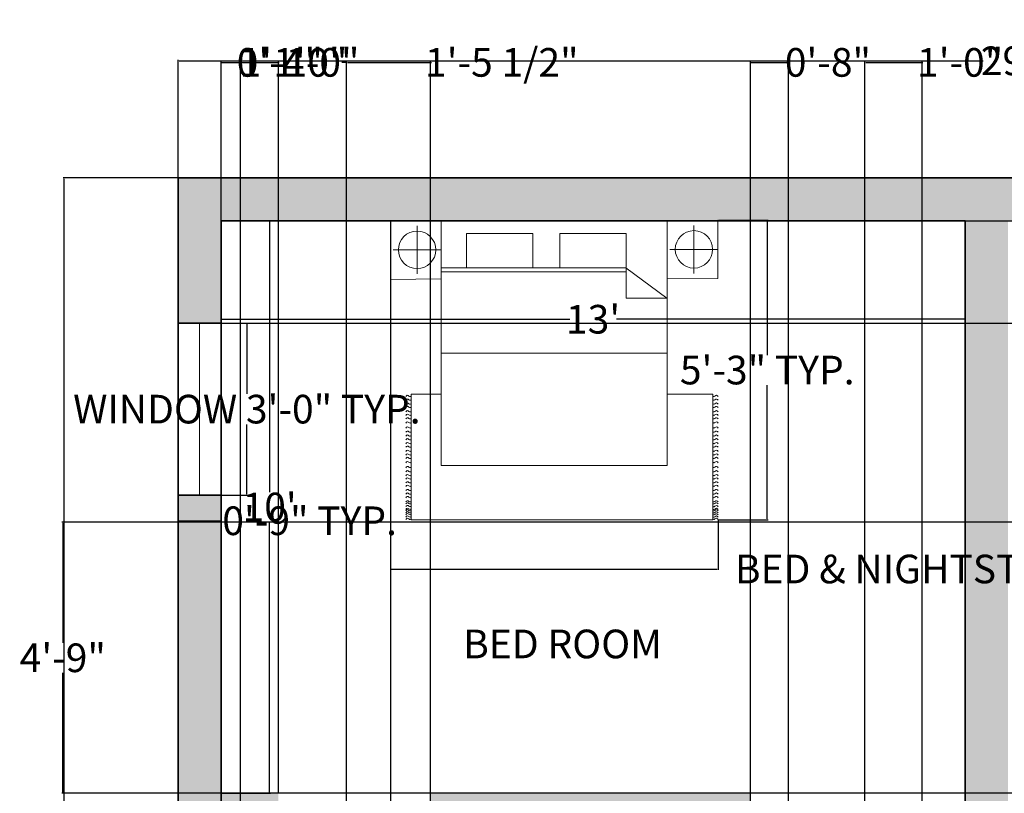
# Model space of a CAD drawing. Units: inches. Extents: x 1174 to 1615, y 3112 to 3628.
# Tile 4 of 6: x 1183 to 1390, y 3466 to 3628. Entities that reach past the tile are written whole.
import ezdxf

# ---------------------------------------------------------------- set-up
doc = ezdxf.new("R2010")
doc.units = ezdxf.units.IN
doc.header["$MEASUREMENT"] = 0
doc.layers.get('0').update_dxf_attribs({"color": 250})
for name, color, linetype, lineweight in [('A-ANNO-DIMS', 2, 'Continuous', 18), ('A-AREA-IDEN', 7, 'Continuous', 25), ('A-FURN', 8, 'Continuous', 13), ('A-GLAZ', 4, 'Continuous', 18), ('A-WALL', 7, 'Continuous', 35)]:
    doc.layers.add(name, color=color, linetype=linetype, lineweight=lineweight)
doc.layers.add('A-WALL-PATT', color=18, linetype='Continuous', lineweight=13, true_color=0x000000)
doc.styles.get("Standard").update_dxf_attribs({"font": 'arial.ttf'})
doc.dimstyles.get("Standard").update_dxf_attribs({"dimtxt": 6, "dimasz": 0.18, "dimexe": 0.18, "dimexo": 0.0625, "dimgap": 0.09, "dimtad": 0, "dimtih": 1, "dimtoh": 1, "dimdec": 1, "dimzin": 0, "dimdsep": 46, "dimlunit": 3, "dimtxsty": 'Standard', "dimcen": 0.09, "dimadec": 0, "dimazin": 0, "dimtfac": 1, "dimtdec": 1, "dimtofl": 0, "dimtmove": 0, "dimatfit": 3, "dimfxl": 1, "dimtolj": 1, "dimtzin": 0, "dimarcsym": 0})

# ---------------------------------------------------------------- blocks, each defined once
blk = doc.blocks.new('*D3')
at = {"layer": 'A-ANNO-DIMS', "color": 0, "lineweight": -2, "transparency": 16777216}
for p, q in [((1216.66, 3595.09), (1216.66, 3619.74)), ((1216.84, 3619.56), (1385.43, 3619.56)), ((1564.48, 3619.56), (1395.9, 3619.56)), ((1564.66, 3595.09), (1564.66, 3619.74))]:
    blk.add_line(p, q, dxfattribs=at)
at = {"layer": 'A-ANNO-DIMS', "color": 0, "transparency": 16777216}
for points in [[(1216.84, 3619.59), (1216.84, 3619.53), (1216.66, 3619.56)], [(1564.48, 3619.59), (1564.48, 3619.53), (1564.66, 3619.56)]]:
    blk.add_solid(points, dxfattribs=at)
at = {"layer": 'Defpoints', "color": 0, "transparency": 16777216}
for p in [(1564.66, 3619.56), (1216.66, 3595.03), (1564.66, 3595.03)]:
    blk.add_point(p, dxfattribs=at)
at = {"layer": 'A-ANNO-DIMS', "color": 0, "transparency": 16777216, "insert": (1390.66, 3619.56), "char_height": 6, "attachment_point": 5}
blk.add_mtext("\\A1;29'", dxfattribs=at)
blk = doc.blocks.new('*D4')
at = {"layer": 'A-ANNO-DIMS', "color": 0, "lineweight": -2, "transparency": 16777216}
for p, q in [((1216.6, 3595.03), (1192.51, 3595.03)), ((1192.69, 3594.85), (1192.69, 3388.18)), ((1192.69, 3175.21), (1192.69, 3381.87)), ((1216.6, 3175.03), (1192.51, 3175.03))]:
    blk.add_line(p, q, dxfattribs=at)
at = {"layer": 'A-ANNO-DIMS', "color": 0, "transparency": 16777216}
for points in [[(1192.66, 3594.85), (1192.72, 3594.85), (1192.69, 3595.03)], [(1192.66, 3175.21), (1192.72, 3175.21), (1192.69, 3175.03)]]:
    blk.add_solid(points, dxfattribs=at)
at = {"layer": 'Defpoints', "color": 0, "transparency": 16777216}
for p in [(1216.66, 3595.03), (1192.69, 3175.03), (1216.66, 3175.03)]:
    blk.add_point(p, dxfattribs=at)
at = {"layer": 'A-ANNO-DIMS', "color": 0, "transparency": 16777216, "insert": (1192.69, 3385.03), "char_height": 6, "attachment_point": 5}
blk.add_mtext("\\A1;35'", dxfattribs=at)
blk = doc.blocks.new('*D5')
at = {"layer": 'A-ANNO-DIMS', "color": 0, "lineweight": -2, "transparency": 16777216}
for p, q in [((1225.73, 3586.03), (1236.02, 3586.03)), ((1235.84, 3585.85), (1235.84, 3529.18)), ((1235.84, 3466.21), (1235.84, 3522.88)), ((1225.73, 3466.03), (1236.02, 3466.03))]:
    blk.add_line(p, q, dxfattribs=at)
at = {"layer": 'A-ANNO-DIMS', "color": 0, "transparency": 16777216}
for points in [[(1235.81, 3585.85), (1235.87, 3585.85), (1235.84, 3586.03)], [(1235.81, 3466.21), (1235.87, 3466.21), (1235.84, 3466.03)]]:
    blk.add_solid(points, dxfattribs=at)
at = {"layer": 'Defpoints', "color": 0, "transparency": 16777216}
for p in [(1225.66, 3586.03), (1225.66, 3466.03), (1235.84, 3466.03)]:
    blk.add_point(p, dxfattribs=at)
at = {"layer": 'A-ANNO-DIMS', "color": 0, "transparency": 16777216, "insert": (1235.84, 3526.03), "char_height": 6, "attachment_point": 5}
blk.add_mtext("\\A1;10'", dxfattribs=at)
blk = doc.blocks.new('*D6')
at = {"layer": 'A-ANNO-DIMS', "color": 0, "lineweight": -2, "transparency": 16777216}
for p, q in [((1225.66, 3585.97), (1225.66, 3565.21)), ((1381.66, 3585.97), (1381.66, 3565.21)), ((1225.84, 3565.39), (1298.76, 3565.39)), ((1381.48, 3565.39), (1308.56, 3565.39))]:
    blk.add_line(p, q, dxfattribs=at)
at = {"layer": 'A-ANNO-DIMS', "color": 0, "transparency": 16777216}
for points in [[(1225.84, 3565.42), (1225.84, 3565.36), (1225.66, 3565.39)], [(1381.48, 3565.42), (1381.48, 3565.36), (1381.66, 3565.39)]]:
    blk.add_solid(points, dxfattribs=at)
at = {"layer": 'Defpoints', "color": 0, "transparency": 16777216}
for p in [(1225.66, 3586.03), (1381.66, 3586.03), (1381.66, 3565.39)]:
    blk.add_point(p, dxfattribs=at)
at = {"layer": 'A-ANNO-DIMS', "color": 0, "transparency": 16777216, "insert": (1303.66, 3565.39), "char_height": 6, "attachment_point": 5}
blk.add_mtext("\\A1;13'", dxfattribs=at)
blk = doc.blocks.new('BED-DOUBLE-WITH-NIGHTSTANDS')
for p, q in [((5.6, 61.61), (5.6, 51.56)), ((63.65, 61.72), (63.65, 51.66)), ((10.63, 56.59), (0.57, 56.59)), ((68.68, 56.69), (58.62, 56.69)), ((49.39, 52.82), (10.63, 52.82)), ((49.44, 52), (10.63, 52)), ((49.39, 52.82), (58, 46.47)), ((49.44, 52.82), (49.44, 46.47)), ((49.44, 46.47), (58, 46.47)), ((58.05, 34.96), (10.63, 34.96)), ((4.35, 0), (4.35, 26.37)), ((4.35, 26.37), (10.65, 26.37)), ((58.05, 26.37), (67.59, 26.37)), ((67.59, 26.37), (67.59, 0)), ((67.59, 0), (4.35, 0))]:
    blk.add_line(p, q)
for points in [[(0, 50.39), (10.63, 50.5), (10.63, 62.68), (0, 62.58)], [(58.05, 62.68), (58.05, 11.36), (10.63, 11.36), (10.63, 62.68)], [(58.05, 50.5), (68.68, 50.6), (68.68, 62.78), (58.05, 62.68)], [(29.88, 59.98), (29.88, 52.82), (15.98, 52.82), (15.98, 59.98)], [(49.44, 59.98), (49.44, 52.82), (35.55, 52.82), (35.55, 59.98)]]:
    blk.add_lwpolyline(points, close=True)
for centre in [(5.6, 56.59), (63.65, 56.69)]:
    blk.add_circle(centre, 3.92)
for points, knots in [([(3.23, 25.83), (3.32, 25.96), (3.52, 26.2), (3.86, 25.96), (4.14, 25.78), (4.29, 25.89), (4.35, 25.94)], [0, 0, 0, 0, 0.400747, 0.791423, 1.067667, 1.29709, 1.29709, 1.29709, 1.29709]), ([(3.23, 25.06), (3.32, 25.18), (3.52, 25.42), (3.86, 25.18), (4.14, 25.01), (4.29, 25.11), (4.35, 25.16)], [0, 0, 0, 0, 0.400747, 0.791423, 1.067667, 1.29709, 1.29709, 1.29709, 1.29709]), ([(68.71, 25.83), (68.61, 25.96), (68.42, 26.2), (68.08, 25.96), (67.8, 25.78), (67.65, 25.89), (67.58, 25.94)], [0, 0, 0, 0, 0.400747, 0.791423, 1.067667, 1.29709, 1.29709, 1.29709, 1.29709]), ([(68.71, 25.06), (68.61, 25.18), (68.42, 25.42), (68.08, 25.18), (67.8, 25.01), (67.65, 25.11), (67.58, 25.16)], [0, 0, 0, 0, 0.400747, 0.791423, 1.067667, 1.29709, 1.29709, 1.29709, 1.29709]), ([(3.23, 24.24), (3.32, 24.36), (3.52, 24.6), (3.86, 24.36), (4.14, 24.19), (4.29, 24.3), (4.35, 24.34)], [0, 0, 0, 0, 0.400747, 0.791423, 1.067667, 1.29709, 1.29709, 1.29709, 1.29709]), ([(3.23, 23.51), (3.32, 23.63), (3.52, 23.87), (3.86, 23.63), (4.14, 23.46), (4.29, 23.57), (4.35, 23.62)], [0, 0, 0, 0, 0.400747, 0.791423, 1.067667, 1.29709, 1.29709, 1.29709, 1.29709]), ([(3.23, 22.63), (3.32, 22.75), (3.52, 22.99), (3.86, 22.75), (4.14, 22.58), (4.29, 22.69), (4.35, 22.73)], [0, 0, 0, 0, 0.400747, 0.791423, 1.067667, 1.29709, 1.29709, 1.29709, 1.29709]), ([(68.71, 24.24), (68.61, 24.36), (68.42, 24.6), (68.08, 24.36), (67.8, 24.19), (67.65, 24.3), (67.58, 24.34)], [0, 0, 0, 0, 0.400747, 0.791423, 1.067667, 1.29709, 1.29709, 1.29709, 1.29709]), ([(68.71, 23.51), (68.61, 23.63), (68.42, 23.87), (68.08, 23.63), (67.8, 23.46), (67.65, 23.57), (67.58, 23.62)], [0, 0, 0, 0, 0.400747, 0.791423, 1.067667, 1.29709, 1.29709, 1.29709, 1.29709]), ([(68.71, 22.63), (68.61, 22.75), (68.42, 22.99), (68.08, 22.75), (67.8, 22.58), (67.65, 22.69), (67.58, 22.73)], [0, 0, 0, 0, 0.400747, 0.791423, 1.067667, 1.29709, 1.29709, 1.29709, 1.29709]), ([(3.23, 21.88), (3.32, 22), (3.52, 22.24), (3.86, 22), (4.14, 21.83), (4.29, 21.93), (4.35, 21.98)], [0, 0, 0, 0, 0.400747, 0.791423, 1.067667, 1.29709, 1.29709, 1.29709, 1.29709]), ([(3.23, 21.15), (3.32, 21.27), (3.52, 21.51), (3.86, 21.27), (4.14, 21.1), (4.29, 21.21), (4.35, 21.25)], [0, 0, 0, 0, 0.400747, 0.791423, 1.067667, 1.29709, 1.29709, 1.29709, 1.29709]), ([(68.71, 21.88), (68.61, 22), (68.42, 22.24), (68.08, 22), (67.8, 21.83), (67.65, 21.93), (67.58, 21.98)], [0, 0, 0, 0, 0.400747, 0.791423, 1.067667, 1.29709, 1.29709, 1.29709, 1.29709]), ([(68.71, 21.15), (68.61, 21.27), (68.42, 21.51), (68.08, 21.27), (67.8, 21.1), (67.65, 21.21), (67.58, 21.25)], [0, 0, 0, 0, 0.400747, 0.791423, 1.067667, 1.29709, 1.29709, 1.29709, 1.29709]), ([(3.23, 20.27), (3.32, 20.39), (3.52, 20.63), (3.86, 20.39), (4.14, 20.22), (4.29, 20.32), (4.35, 20.37)], [0, 0, 0, 0, 0.400747, 0.791423, 1.067667, 1.29709, 1.29709, 1.29709, 1.29709]), ([(3.23, 19.23), (3.32, 19.35), (3.52, 19.59), (3.86, 19.35), (4.14, 19.18), (4.29, 19.29), (4.35, 19.33)], [0, 0, 0, 0, 0.400747, 0.791423, 1.067667, 1.29709, 1.29709, 1.29709, 1.29709]), ([(3.23, 18.35), (3.32, 18.47), (3.52, 18.71), (3.86, 18.47), (4.14, 18.3), (4.29, 18.4), (4.35, 18.45)], [0, 0, 0, 0, 0.400747, 0.791423, 1.067667, 1.29709, 1.29709, 1.29709, 1.29709]), ([(68.71, 20.27), (68.61, 20.39), (68.42, 20.63), (68.08, 20.39), (67.8, 20.22), (67.65, 20.32), (67.58, 20.37)], [0, 0, 0, 0, 0.400747, 0.791423, 1.067667, 1.29709, 1.29709, 1.29709, 1.29709]), ([(68.71, 19.23), (68.61, 19.35), (68.42, 19.59), (68.08, 19.35), (67.8, 19.18), (67.65, 19.29), (67.58, 19.33)], [0, 0, 0, 0, 0.400747, 0.791423, 1.067667, 1.29709, 1.29709, 1.29709, 1.29709]), ([(68.71, 18.35), (68.61, 18.47), (68.42, 18.71), (68.08, 18.47), (67.8, 18.3), (67.65, 18.4), (67.58, 18.45)], [0, 0, 0, 0, 0.400747, 0.791423, 1.067667, 1.29709, 1.29709, 1.29709, 1.29709]), ([(3.23, 17.53), (3.32, 17.65), (3.52, 17.89), (3.86, 17.65), (4.14, 17.48), (4.29, 17.59), (4.35, 17.64)], [0, 0, 0, 0, 0.400747, 0.791423, 1.067667, 1.29709, 1.29709, 1.29709, 1.29709]), ([(3.23, 16.76), (3.32, 16.88), (3.52, 17.12), (3.86, 16.88), (4.14, 16.7), (4.29, 16.81), (4.35, 16.86)], [0, 0, 0, 0, 0.400747, 0.791423, 1.067667, 1.29709, 1.29709, 1.29709, 1.29709]), ([(68.71, 17.53), (68.61, 17.65), (68.42, 17.89), (68.08, 17.65), (67.8, 17.48), (67.65, 17.59), (67.58, 17.64)], [0, 0, 0, 0, 0.400747, 0.791423, 1.067667, 1.29709, 1.29709, 1.29709, 1.29709]), ([(68.71, 16.76), (68.61, 16.88), (68.42, 17.12), (68.08, 16.88), (67.8, 16.7), (67.65, 16.81), (67.58, 16.86)], [0, 0, 0, 0, 0.400747, 0.791423, 1.067667, 1.29709, 1.29709, 1.29709, 1.29709]), ([(3.23, 15.94), (3.32, 16.06), (3.52, 16.3), (3.86, 16.06), (4.14, 15.89), (4.29, 15.99), (4.35, 16.04)], [0, 0, 0, 0, 0.400747, 0.791423, 1.067667, 1.29709, 1.29709, 1.29709, 1.29709]), ([(3.23, 15.21), (3.32, 15.33), (3.52, 15.57), (3.86, 15.33), (4.14, 15.16), (4.29, 15.27), (4.35, 15.32)], [0, 0, 0, 0, 0.400747, 0.791423, 1.067667, 1.29709, 1.29709, 1.29709, 1.29709]), ([(3.23, 14.33), (3.32, 14.45), (3.52, 14.69), (3.86, 14.45), (4.14, 14.28), (4.29, 14.38), (4.35, 14.43)], [0, 0, 0, 0, 0.400747, 0.791423, 1.067667, 1.29709, 1.29709, 1.29709, 1.29709]), ([(68.71, 15.94), (68.61, 16.06), (68.42, 16.3), (68.08, 16.06), (67.8, 15.89), (67.65, 15.99), (67.58, 16.04)], [0, 0, 0, 0, 0.400747, 0.791423, 1.067667, 1.29709, 1.29709, 1.29709, 1.29709]), ([(68.71, 15.21), (68.61, 15.33), (68.42, 15.57), (68.08, 15.33), (67.8, 15.16), (67.65, 15.27), (67.58, 15.32)], [0, 0, 0, 0, 0.400747, 0.791423, 1.067667, 1.29709, 1.29709, 1.29709, 1.29709]), ([(68.71, 14.33), (68.61, 14.45), (68.42, 14.69), (68.08, 14.45), (67.8, 14.28), (67.65, 14.38), (67.58, 14.43)], [0, 0, 0, 0, 0.400747, 0.791423, 1.067667, 1.29709, 1.29709, 1.29709, 1.29709]), ([(3.23, 13.58), (3.32, 13.7), (3.52, 13.94), (3.86, 13.7), (4.14, 13.53), (4.29, 13.63), (4.35, 13.68)], [0, 0, 0, 0, 0.400747, 0.791423, 1.067667, 1.29709, 1.29709, 1.29709, 1.29709]), ([(3.23, 12.85), (3.32, 12.97), (3.52, 13.21), (3.86, 12.97), (4.14, 12.8), (4.29, 12.9), (4.35, 12.95)], [0, 0, 0, 0, 0.400747, 0.791423, 1.067667, 1.29709, 1.29709, 1.29709, 1.29709]), ([(68.71, 13.58), (68.61, 13.7), (68.42, 13.94), (68.08, 13.7), (67.8, 13.53), (67.65, 13.63), (67.58, 13.68)], [0, 0, 0, 0, 0.400747, 0.791423, 1.067667, 1.29709, 1.29709, 1.29709, 1.29709]), ([(68.71, 12.85), (68.61, 12.97), (68.42, 13.21), (68.08, 12.97), (67.8, 12.8), (67.65, 12.9), (67.58, 12.95)], [0, 0, 0, 0, 0.400747, 0.791423, 1.067667, 1.29709, 1.29709, 1.29709, 1.29709]), ([(3.23, 11.97), (3.32, 12.09), (3.52, 12.33), (3.86, 12.09), (4.14, 11.92), (4.29, 12.02), (4.35, 12.07)], [0, 0, 0, 0, 0.400747, 0.791423, 1.067667, 1.29709, 1.29709, 1.29709, 1.29709]), ([(3.23, 10.93), (3.32, 11.05), (3.52, 11.29), (3.86, 11.05), (4.14, 10.88), (4.29, 10.99), (4.35, 11.03)], [0, 0, 0, 0, 0.400747, 0.791423, 1.067667, 1.29709, 1.29709, 1.29709, 1.29709]), ([(68.71, 11.97), (68.61, 12.09), (68.42, 12.33), (68.08, 12.09), (67.8, 11.92), (67.65, 12.02), (67.58, 12.07)], [0, 0, 0, 0, 0.400747, 0.791423, 1.067667, 1.29709, 1.29709, 1.29709, 1.29709]), ([(68.71, 10.93), (68.61, 11.05), (68.42, 11.29), (68.08, 11.05), (67.8, 10.88), (67.65, 10.99), (67.58, 11.03)], [0, 0, 0, 0, 0.400747, 0.791423, 1.067667, 1.29709, 1.29709, 1.29709, 1.29709]), ([(3.23, 10.05), (3.32, 10.17), (3.52, 10.41), (3.86, 10.17), (4.14, 10), (4.29, 10.1), (4.35, 10.15)], [0, 0, 0, 0, 0.400747, 0.791423, 1.067667, 1.29709, 1.29709, 1.29709, 1.29709]), ([(3.23, 9.23), (3.32, 9.35), (3.52, 9.59), (3.86, 9.35), (4.14, 9.18), (4.29, 9.29), (4.35, 9.34)], [0, 0, 0, 0, 0.400747, 0.791423, 1.067667, 1.29709, 1.29709, 1.29709, 1.29709]), ([(3.23, 8.54), (3.32, 8.66), (3.52, 8.9), (3.86, 8.66), (4.14, 8.49), (4.29, 8.6), (4.35, 8.65)], [0, 0, 0, 0, 0.400747, 0.791423, 1.067667, 1.29709, 1.29709, 1.29709, 1.29709]), ([(68.71, 10.05), (68.61, 10.17), (68.42, 10.41), (68.08, 10.17), (67.8, 10), (67.65, 10.1), (67.58, 10.15)], [0, 0, 0, 0, 0.400747, 0.791423, 1.067667, 1.29709, 1.29709, 1.29709, 1.29709]), ([(68.71, 9.23), (68.61, 9.35), (68.42, 9.59), (68.08, 9.35), (67.8, 9.18), (67.65, 9.29), (67.58, 9.34)], [0, 0, 0, 0, 0.400747, 0.791423, 1.067667, 1.29709, 1.29709, 1.29709, 1.29709]), ([(68.71, 8.54), (68.61, 8.66), (68.42, 8.9), (68.08, 8.66), (67.8, 8.49), (67.65, 8.6), (67.58, 8.65)], [0, 0, 0, 0, 0.400747, 0.791423, 1.067667, 1.29709, 1.29709, 1.29709, 1.29709]), ([(3.23, 7.73), (3.32, 7.85), (3.52, 8.09), (3.86, 7.85), (4.14, 7.68), (4.29, 7.78), (4.35, 7.83)], [0, 0, 0, 0, 0.400747, 0.791423, 1.067667, 1.29709, 1.29709, 1.29709, 1.29709]), ([(3.23, 7), (3.32, 7.12), (3.52, 7.36), (3.86, 7.12), (4.14, 6.95), (4.29, 7.05), (4.35, 7.1)], [0, 0, 0, 0, 0.400747, 0.791423, 1.067667, 1.29709, 1.29709, 1.29709, 1.29709]), ([(3.23, 6.12), (3.32, 6.24), (3.52, 6.48), (3.86, 6.24), (4.14, 6.06), (4.29, 6.17), (4.35, 6.22)], [0, 0, 0, 0, 0.400747, 0.791423, 1.067667, 1.29709, 1.29709, 1.29709, 1.29709]), ([(68.71, 7.73), (68.61, 7.85), (68.42, 8.09), (68.08, 7.85), (67.8, 7.68), (67.65, 7.78), (67.58, 7.83)], [0, 0, 0, 0, 0.400747, 0.791423, 1.067667, 1.29709, 1.29709, 1.29709, 1.29709]), ([(68.71, 7), (68.61, 7.12), (68.42, 7.36), (68.08, 7.12), (67.8, 6.95), (67.65, 7.05), (67.58, 7.1)], [0, 0, 0, 0, 0.400747, 0.791423, 1.067667, 1.29709, 1.29709, 1.29709, 1.29709]), ([(68.71, 6.12), (68.61, 6.24), (68.42, 6.48), (68.08, 6.24), (67.8, 6.06), (67.65, 6.17), (67.58, 6.22)], [0, 0, 0, 0, 0.400747, 0.791423, 1.067667, 1.29709, 1.29709, 1.29709, 1.29709]), ([(3.23, 5.36), (3.32, 5.49), (3.52, 5.73), (3.86, 5.49), (4.14, 5.31), (4.29, 5.42), (4.35, 5.47)], [0, 0, 0, 0, 0.400747, 0.791423, 1.067667, 1.29709, 1.29709, 1.29709, 1.29709]), ([(3.23, 4.64), (3.32, 4.76), (3.52, 5), (3.86, 4.76), (4.14, 4.58), (4.29, 4.69), (4.35, 4.74)], [0, 0, 0, 0, 0.400747, 0.791423, 1.067667, 1.29709, 1.29709, 1.29709, 1.29709]), ([(68.71, 5.36), (68.61, 5.49), (68.42, 5.73), (68.08, 5.49), (67.8, 5.31), (67.65, 5.42), (67.58, 5.47)], [0, 0, 0, 0, 0.400747, 0.791423, 1.067667, 1.29709, 1.29709, 1.29709, 1.29709]), ([(68.71, 4.64), (68.61, 4.76), (68.42, 5), (68.08, 4.76), (67.8, 4.59), (67.66, 4.69), (67.59, 4.73)], [0, 0, 0, 0, 0.400747, 0.791423, 1.067667, 1.283686, 1.283686, 1.283686, 1.283686]), ([(3.23, 3.75), (3.32, 3.88), (3.52, 4.11), (3.86, 3.88), (4.14, 3.7), (4.29, 3.81), (4.35, 3.86)], [0, 0, 0, 0, 0.400747, 0.791423, 1.067667, 1.29709, 1.29709, 1.29709, 1.29709]), ([(3.23, 3.32), (3.32, 3.45), (3.51, 3.7), (3.86, 3.44), (4.14, 3.27), (4.29, 3.38), (4.35, 3.43)], [0, 0, 0, 0, 0.407265, 0.802015, 1.07826, 1.307683, 1.307683, 1.307683, 1.307683]), ([(3.23, 2.76), (3.32, 2.88), (3.52, 3.12), (3.86, 2.88), (4.14, 2.71), (4.29, 2.81), (4.35, 2.86)], [0, 0, 0, 0, 0.400747, 0.791423, 1.067667, 1.29709, 1.29709, 1.29709, 1.29709]), ([(3.23, 2.18), (3.32, 2.31), (3.52, 2.55), (3.86, 2.31), (4.14, 2.13), (4.29, 2.24), (4.35, 2.29)], [0, 0, 0, 0, 0.400747, 0.791423, 1.067667, 1.29709, 1.29709, 1.29709, 1.29709]), ([(3.23, 1.88), (3.32, 2), (3.52, 2.24), (3.86, 2), (4.14, 1.82), (4.29, 1.93), (4.35, 1.98)], [0, 0, 0, 0, 0.400747, 0.791423, 1.067667, 1.29709, 1.29709, 1.29709, 1.29709]), ([(68.71, 3.75), (68.61, 3.88), (68.42, 4.11), (68.08, 3.88), (67.8, 3.7), (67.66, 3.8), (67.59, 3.85)], [0, 0, 0, 0, 0.400747, 0.791423, 1.067667, 1.283686, 1.283686, 1.283686, 1.283686]), ([(68.71, 3.32), (68.61, 3.45), (68.42, 3.69), (68.08, 3.45), (67.8, 3.27), (67.66, 3.38), (67.59, 3.42)], [0, 0, 0, 0, 0.402903, 0.794912, 1.071156, 1.287177, 1.287177, 1.287177, 1.287177]), ([(68.71, 2.73), (68.61, 2.85), (68.42, 3.09), (68.08, 2.85), (67.8, 2.68), (67.66, 2.78), (67.59, 2.82)], [0, 0, 0, 0, 0.400747, 0.791423, 1.067667, 1.283686, 1.283686, 1.283686, 1.283686]), ([(68.71, 2.16), (68.61, 2.28), (68.42, 2.52), (68.08, 2.28), (67.8, 2.11), (67.66, 2.21), (67.59, 2.25)], [0, 0, 0, 0, 0.400747, 0.791423, 1.067667, 1.283686, 1.283686, 1.283686, 1.283686]), ([(68.71, 1.85), (68.61, 1.97), (68.42, 2.21), (68.08, 1.97), (67.8, 1.8), (67.66, 1.9), (67.59, 1.94)], [0, 0, 0, 0, 0.400747, 0.791423, 1.067667, 1.283686, 1.283686, 1.283686, 1.283686]), ([(3.23, 1.46), (3.32, 1.58), (3.52, 1.82), (3.86, 1.58), (4.14, 1.4), (4.29, 1.51), (4.35, 1.56)], [0, 0, 0, 0, 0.400747, 0.791423, 1.067667, 1.29709, 1.29709, 1.29709, 1.29709]), ([(3.23, 1.06), (3.32, 1.18), (3.52, 1.42), (3.86, 1.18), (4.14, 1.01), (4.29, 1.11), (4.35, 1.16)], [0, 0, 0, 0, 0.400747, 0.791423, 1.067667, 1.29709, 1.29709, 1.29709, 1.29709]), ([(3.23, 0.57), (3.32, 0.7), (3.52, 0.93), (3.86, 0.7), (4.14, 0.52), (4.29, 0.63), (4.35, 0.68)], [0, 0, 0, 0, 0.400747, 0.791423, 1.067667, 1.29709, 1.29709, 1.29709, 1.29709]), ([(3.23, 0.07), (3.32, 0.19), (3.52, 0.43), (3.86, 0.19), (4.14, 0.02), (4.29, 0.13), (4.35, 0.18)], [0, 0, 0, 0, 0.400747, 0.791423, 1.067667, 1.29709, 1.29709, 1.29709, 1.29709]), ([(68.71, 1.43), (68.61, 1.55), (68.42, 1.79), (68.08, 1.55), (67.8, 1.38), (67.65, 1.48), (67.58, 1.53)], [0, 0, 0, 0, 0.400747, 0.791423, 1.067667, 1.29709, 1.29709, 1.29709, 1.29709]), ([(68.71, 1.03), (68.61, 1.15), (68.42, 1.39), (68.08, 1.15), (67.8, 0.98), (67.65, 1.09), (67.58, 1.13)], [0, 0, 0, 0, 0.400747, 0.791423, 1.067667, 1.29709, 1.29709, 1.29709, 1.29709]), ([(68.71, 0.55), (68.61, 0.67), (68.42, 0.91), (68.08, 0.67), (67.8, 0.49), (67.65, 0.6), (67.58, 0.65)], [0, 0, 0, 0, 0.400747, 0.791423, 1.067667, 1.29709, 1.29709, 1.29709, 1.29709]), ([(68.71, 0.07), (68.61, 0.19), (68.42, 0.43), (68.08, 0.19), (67.8, 0.02), (67.65, 0.13), (67.58, 0.18)], [0, 0, 0, 0, 0.400747, 0.791423, 1.067667, 1.29709, 1.29709, 1.29709, 1.29709])]:
    blk.add_open_spline(points, degree=3, knots=knots)
blk = doc.blocks.new('WINDOW-36IN')
for p, q in [((-4.5, -36), (-4.5, 0)), ((0, 0), (0, -36)), ((4.5, 0), (4.5, -36))]:
    blk.add_line(p, q)
blk = doc.blocks.new('*D26')
at = {"layer": 'A-ANNO-DIMS', "color": 0, "lineweight": -2, "transparency": 16777216}
for p, q in [((1225.73, 3564.55), (1231.24, 3564.55)), ((1231.06, 3564.37), (1231.06, 3549.75)), ((1231.06, 3528.73), (1231.06, 3543.36)), ((1225.73, 3528.55), (1231.24, 3528.55))]:
    blk.add_line(p, q, dxfattribs=at)
at = {"layer": 'A-ANNO-DIMS', "color": 0, "transparency": 16777216}
for points in [[(1231.03, 3564.37), (1231.09, 3564.37), (1231.06, 3564.55)], [(1231.03, 3528.73), (1231.09, 3528.73), (1231.06, 3528.55)]]:
    blk.add_solid(points, dxfattribs=at)
at = {"layer": 'Defpoints', "color": 0, "transparency": 16777216}
for p in [(1225.66, 3564.55), (1231.06, 3564.55), (1225.66, 3528.55)]:
    blk.add_point(p, dxfattribs=at)
at = {"layer": 'A-ANNO-DIMS', "color": 0, "transparency": 16777216, "insert": (1231.06, 3546.55), "char_height": 6, "attachment_point": 5}
blk.add_mtext('\\A1;WINDOW 3\'-0" TYP.', dxfattribs=at)
blk = doc.blocks.new('*D27')
at = {"layer": 'A-ANNO-DIMS', "color": 0, "lineweight": -2, "transparency": 16777216}
for p, q in [((1216.66, 3528.49), (1216.66, 3522.97)), ((1225.66, 3528.49), (1225.66, 3522.97)), ((1216.84, 3523.15), (1225.48, 3523.15)), ((1225.66, 3523.15), (1225.84, 3523.15))]:
    blk.add_line(p, q, dxfattribs=at)
at = {"layer": 'A-ANNO-DIMS', "color": 0, "transparency": 16777216}
for points in [[(1216.84, 3523.18), (1216.84, 3523.12), (1216.66, 3523.15)], [(1225.48, 3523.18), (1225.48, 3523.12), (1225.66, 3523.15)]]:
    blk.add_solid(points, dxfattribs=at)
at = {"layer": 'Defpoints', "color": 0, "transparency": 16777216}
for p in [(1216.66, 3528.55), (1225.66, 3528.55), (1225.66, 3523.15)]:
    blk.add_point(p, dxfattribs=at)
at = {"layer": 'A-ANNO-DIMS', "color": 0, "transparency": 16777216, "insert": (1244.22, 3523.15), "char_height": 6, "attachment_point": 5}
blk.add_mtext('\\A1;0\'-9" TYP.', dxfattribs=at)
blk = doc.blocks.new('*D30')
at = {"layer": 'A-ANNO-DIMS', "color": 0, "lineweight": -2, "transparency": 16777216}
for p, q in [((1261.16, 3523.29), (1261.16, 3512.86)), ((1329.87, 3523.29), (1329.87, 3512.86)), ((1261.34, 3513.04), (1329.69, 3513.04)), ((1329.87, 3513.04), (1330.05, 3513.04))]:
    blk.add_line(p, q, dxfattribs=at)
at = {"layer": 'A-ANNO-DIMS', "color": 0, "transparency": 16777216}
for points in [[(1261.34, 3513.07), (1261.34, 3513.01), (1261.16, 3513.04)], [(1329.69, 3513.07), (1329.69, 3513.01), (1329.87, 3513.04)]]:
    blk.add_solid(points, dxfattribs=at)
at = {"layer": 'Defpoints', "color": 0, "transparency": 16777216}
for p in [(1261.16, 3523.35), (1329.87, 3523.35), (1329.87, 3513.04)]:
    blk.add_point(p, dxfattribs=at)
at = {"layer": 'A-ANNO-DIMS', "color": 0, "transparency": 16777216, "insert": (1400.23, 3513.04), "char_height": 6, "attachment_point": 5}
blk.add_mtext('\\A1;BED & NIGHTSTANDS 5\'-8 1/2" TYP.', dxfattribs=at)
blk = doc.blocks.new('*D31')
at = {"layer": 'A-ANNO-DIMS', "color": 0, "lineweight": -2, "transparency": 16777216}
for p, q in [((1329.94, 3586.13), (1340.36, 3586.13)), ((1340.18, 3585.95), (1340.18, 3557.89)), ((1340.18, 3523.53), (1340.18, 3551.58)), ((1329.94, 3523.35), (1340.36, 3523.35))]:
    blk.add_line(p, q, dxfattribs=at)
at = {"layer": 'A-ANNO-DIMS', "color": 0, "transparency": 16777216}
for points in [[(1340.15, 3585.95), (1340.21, 3585.95), (1340.18, 3586.13)], [(1340.15, 3523.53), (1340.21, 3523.53), (1340.18, 3523.35)]]:
    blk.add_solid(points, dxfattribs=at)
at = {"layer": 'Defpoints', "color": 0, "transparency": 16777216}
for p in [(1329.87, 3586.13), (1340.18, 3586.13), (1329.87, 3523.35)]:
    blk.add_point(p, dxfattribs=at)
at = {"layer": 'A-ANNO-DIMS', "color": 0, "transparency": 16777216, "insert": (1340.18, 3554.74), "char_height": 6, "attachment_point": 5}
blk.add_mtext('\\A1;5\'-3" TYP.', dxfattribs=at)
blk = doc.blocks.new('*D47')
at = {"layer": 'A-ANNO-DIMS', "color": 0, "lineweight": -2, "transparency": 16777216}
for p, q in [((1225.73, 3586.03), (1589.04, 3586.03)), ((1588.86, 3585.85), (1588.86, 3578.48)), ((1588.86, 3564.73), (1588.86, 3572.1)), ((1225.73, 3564.55), (1589.04, 3564.55))]:
    blk.add_line(p, q, dxfattribs=at)
at = {"layer": 'A-ANNO-DIMS', "color": 0, "transparency": 16777216}
for points in [[(1588.83, 3585.85), (1588.89, 3585.85), (1588.86, 3586.03)], [(1588.83, 3564.73), (1588.89, 3564.73), (1588.86, 3564.55)]]:
    blk.add_solid(points, dxfattribs=at)
at = {"layer": 'Defpoints', "color": 0, "transparency": 16777216}
for p in [(1225.66, 3586.03), (1225.66, 3564.55), (1588.86, 3564.55)]:
    blk.add_point(p, dxfattribs=at)
at = {"layer": 'A-ANNO-DIMS', "color": 0, "transparency": 16777216, "insert": (1588.86, 3575.29), "char_height": 6, "attachment_point": 5}
blk.add_mtext('\\A1;1\'-9 1/2"', dxfattribs=at)
blk = doc.blocks.new('*D50')
at = {"layer": 'A-ANNO-DIMS', "color": 0, "lineweight": -2, "transparency": 16777216}
for p, q in [((1555.6, 3522.83), (1192.28, 3522.83)), ((1192.46, 3522.65), (1192.46, 3497.58)), ((1192.46, 3466.21), (1192.46, 3491.28)), ((1555.6, 3466.03), (1192.28, 3466.03))]:
    blk.add_line(p, q, dxfattribs=at)
at = {"layer": 'A-ANNO-DIMS', "color": 0, "transparency": 16777216}
for points in [[(1192.43, 3522.65), (1192.49, 3522.65), (1192.46, 3522.83)], [(1192.43, 3466.21), (1192.49, 3466.21), (1192.46, 3466.03)]]:
    blk.add_solid(points, dxfattribs=at)
at = {"layer": 'Defpoints', "color": 0, "transparency": 16777216}
for p in [(1555.66, 3522.83), (1192.46, 3466.03), (1555.66, 3466.03)]:
    blk.add_point(p, dxfattribs=at)
at = {"layer": 'A-ANNO-DIMS', "color": 0, "transparency": 16777216, "insert": (1192.46, 3494.43), "char_height": 6, "attachment_point": 5}
blk.add_mtext('\\A1;4\'-9"', dxfattribs=at)
blk = doc.blocks.new('*D54')
at = {"layer": 'A-ANNO-DIMS', "color": 0, "lineweight": -2, "transparency": 16777216}
for p, q in [((1225.66, 3466.09), (1225.66, 3619.41)), ((1225.84, 3619.23), (1237.48, 3619.23)), ((1237.66, 3466.09), (1237.66, 3619.41)), ((1237.66, 3619.23), (1237.84, 3619.23))]:
    blk.add_line(p, q, dxfattribs=at)
at = {"layer": 'A-ANNO-DIMS', "color": 0, "transparency": 16777216}
for points in [[(1225.84, 3619.26), (1225.84, 3619.2), (1225.66, 3619.23)], [(1237.48, 3619.26), (1237.48, 3619.2), (1237.66, 3619.23)]]:
    blk.add_solid(points, dxfattribs=at)
at = {"layer": 'Defpoints', "color": 0, "transparency": 16777216}
for p in [(1237.66, 3619.23), (1225.66, 3466.03), (1237.66, 3466.03)]:
    blk.add_point(p, dxfattribs=at)
at = {"layer": 'A-ANNO-DIMS', "color": 0, "transparency": 16777216, "insert": (1245.63, 3619.23), "char_height": 6, "attachment_point": 5}
blk.add_mtext('\\A1;1\'-0"', dxfattribs=at)
blk = doc.blocks.new('*D56')
at = {"layer": 'A-ANNO-DIMS', "color": 0, "lineweight": -2, "transparency": 16777216}
for p, q in [((1336.66, 3385.09), (1336.66, 3619.41)), ((1336.84, 3619.23), (1344.48, 3619.23)), ((1344.66, 3385.09), (1344.66, 3619.41)), ((1344.66, 3619.23), (1344.84, 3619.23))]:
    blk.add_line(p, q, dxfattribs=at)
at = {"layer": 'A-ANNO-DIMS', "color": 0, "transparency": 16777216}
for points in [[(1336.84, 3619.26), (1336.84, 3619.2), (1336.66, 3619.23)], [(1344.48, 3619.26), (1344.48, 3619.2), (1344.66, 3619.23)]]:
    blk.add_solid(points, dxfattribs=at)
at = {"layer": 'Defpoints', "color": 0, "transparency": 16777216}
for p in [(1344.66, 3619.23), (1336.66, 3385.03), (1344.66, 3385.03)]:
    blk.add_point(p, dxfattribs=at)
at = {"layer": 'A-ANNO-DIMS', "color": 0, "transparency": 16777216, "insert": (1352.91, 3619.23), "char_height": 6, "attachment_point": 5}
blk.add_mtext('\\A1;0\'-8"', dxfattribs=at)
blk = doc.blocks.new('*D58')
at = {"layer": 'A-ANNO-DIMS', "color": 0, "lineweight": -2, "transparency": 16777216}
for p, q in [((1360.66, 3184.09), (1360.66, 3619.41)), ((1360.84, 3619.23), (1372.48, 3619.23)), ((1372.66, 3184.09), (1372.66, 3619.41)), ((1372.66, 3619.23), (1372.84, 3619.23))]:
    blk.add_line(p, q, dxfattribs=at)
at = {"layer": 'A-ANNO-DIMS', "color": 0, "transparency": 16777216}
for points in [[(1360.84, 3619.26), (1360.84, 3619.2), (1360.66, 3619.23)], [(1372.48, 3619.26), (1372.48, 3619.2), (1372.66, 3619.23)]]:
    blk.add_solid(points, dxfattribs=at)
at = {"layer": 'Defpoints', "color": 0, "transparency": 16777216}
for p in [(1372.66, 3619.23), (1360.66, 3184.03), (1372.66, 3184.03)]:
    blk.add_point(p, dxfattribs=at)
at = {"layer": 'A-ANNO-DIMS', "color": 0, "transparency": 16777216, "insert": (1380.63, 3619.23), "char_height": 6, "attachment_point": 5}
blk.add_mtext('\\A1;1\'-0"', dxfattribs=at)
blk = doc.blocks.new('*D60')
at = {"layer": 'A-ANNO-DIMS', "color": 0, "lineweight": -2, "transparency": 16777216}
for p, q in [((1229.72, 3290.15), (1229.72, 3619.41)), ((1229.9, 3619.23), (1230.72, 3619.23)), ((1251.77, 3619.23), (1250.95, 3619.23)), ((1251.95, 3292.11), (1251.95, 3619.41))]:
    blk.add_line(p, q, dxfattribs=at)
at = {"layer": 'A-ANNO-DIMS', "color": 0, "transparency": 16777216}
for points in [[(1229.9, 3619.26), (1229.9, 3619.2), (1229.72, 3619.23)], [(1251.77, 3619.26), (1251.77, 3619.2), (1251.95, 3619.23)]]:
    blk.add_solid(points, dxfattribs=at)
at = {"layer": 'Defpoints', "color": 0, "transparency": 16777216}
for p in [(1251.95, 3619.23), (1251.95, 3292.05), (1229.72, 3290.09)]:
    blk.add_point(p, dxfattribs=at)
at = {"layer": 'A-ANNO-DIMS', "color": 0, "transparency": 16777216, "insert": (1240.84, 3619.23), "char_height": 6, "attachment_point": 5}
blk.add_mtext('\\A1;1\'-10"', dxfattribs=at)
blk = doc.blocks.new('*D64')
at = {"layer": 'A-ANNO-DIMS', "color": 0, "lineweight": -2, "transparency": 16777216}
for p, q in [((1251.95, 3292.11), (1251.95, 3619.41)), ((1252.13, 3619.23), (1269.39, 3619.23)), ((1269.57, 3281.81), (1269.57, 3619.41)), ((1269.57, 3619.23), (1269.75, 3619.23))]:
    blk.add_line(p, q, dxfattribs=at)
at = {"layer": 'A-ANNO-DIMS', "color": 0, "transparency": 16777216}
for points in [[(1252.13, 3619.26), (1252.13, 3619.2), (1251.95, 3619.23)], [(1269.39, 3619.26), (1269.39, 3619.2), (1269.57, 3619.23)]]:
    blk.add_solid(points, dxfattribs=at)
at = {"layer": 'Defpoints', "color": 0, "transparency": 16777216}
for p in [(1269.57, 3619.23), (1251.95, 3292.05), (1269.57, 3281.75)]:
    blk.add_point(p, dxfattribs=at)
at = {"layer": 'A-ANNO-DIMS', "color": 0, "transparency": 16777216, "insert": (1284.52, 3619.23), "char_height": 6, "attachment_point": 5}
blk.add_mtext('\\A1;1\'-5 1/2"', dxfattribs=at)
blk = doc.blocks.new('*D69')
at = {"layer": 'A-ANNO-DIMS', "color": 0, "lineweight": -2, "transparency": 16777216}
for p, q in [((1225.66, 3585.97), (1225.66, 3120.65)), ((1261.16, 3585.86), (1261.16, 3120.65)), ((1225.84, 3120.83), (1225.98, 3120.83)), ((1260.98, 3120.83), (1260.85, 3120.83))]:
    blk.add_line(p, q, dxfattribs=at)
at = {"layer": 'A-ANNO-DIMS', "color": 0, "transparency": 16777216}
for points in [[(1225.84, 3120.86), (1225.84, 3120.8), (1225.66, 3120.83)], [(1260.98, 3120.86), (1260.98, 3120.8), (1261.16, 3120.83)]]:
    blk.add_solid(points, dxfattribs=at)
at = {"layer": 'Defpoints', "color": 0, "transparency": 16777216}
for p in [(1225.66, 3586.03), (1261.16, 3585.93), (1261.16, 3120.83)]:
    blk.add_point(p, dxfattribs=at)
at = {"layer": 'A-ANNO-DIMS', "color": 0, "transparency": 16777216, "insert": (1243.41, 3120.83), "char_height": 6, "attachment_point": 5}
blk.add_mtext('\\A1;2\'-11 1/2"', dxfattribs=at)
blk = doc.blocks.new('*D71')
at = {"layer": 'A-ANNO-DIMS', "color": 0, "lineweight": -2, "transparency": 16777216}
for p, q in [((1225.66, 3283.7), (1225.66, 3619.41)), ((1225.84, 3619.23), (1229.54, 3619.23)), ((1229.72, 3290.15), (1229.72, 3619.41)), ((1229.72, 3619.23), (1229.9, 3619.23))]:
    blk.add_line(p, q, dxfattribs=at)
at = {"layer": 'A-ANNO-DIMS', "color": 0, "transparency": 16777216}
for points in [[(1225.84, 3619.26), (1225.84, 3619.2), (1225.66, 3619.23)], [(1229.54, 3619.26), (1229.54, 3619.2), (1229.72, 3619.23)]]:
    blk.add_solid(points, dxfattribs=at)
at = {"layer": 'Defpoints', "color": 0, "transparency": 16777216}
for p in [(1229.72, 3619.23), (1229.72, 3290.09), (1225.66, 3283.63)]:
    blk.add_point(p, dxfattribs=at)
at = {"layer": 'A-ANNO-DIMS', "color": 0, "transparency": 16777216, "insert": (1237.97, 3619.23), "char_height": 6, "attachment_point": 5}
blk.add_mtext('\\A1;0\'-4"', dxfattribs=at)

msp = doc.modelspace()

# ---------------------------------------------------------------- hatches: boundary and pattern name
at = {"layer": 'A-WALL-PATT'}
h = msp.add_hatch(color=256, dxfattribs=at)
h.dxf.hatch_style = 1
h.paths.add_polyline_path([(1564.66, 3595.03), (1216.66, 3595.03), (1216.66, 3564.55), (1225.66, 3564.55), (1225.66, 3586.03), (1381.66, 3586.03), (1381.66, 3385.03), (1380.66, 3385.03), (1380.66, 3376.03), (1381.66, 3376.03), (1407.66, 3376.03), (1407.66, 3385.03), (1390.66, 3385.03), (1390.66, 3586.03), (1555.66, 3586.03), (1555.66, 3558.83), (1564.66, 3558.83)])
h.paths.add_polyline_path([(1564.66, 3408.64), (1555.66, 3408.64), (1555.66, 3385.03), (1453.66, 3385.03), (1453.66, 3457.03), (1465.66, 3457.03), (1465.66, 3466.03), (1453.66, 3466.03), (1444.66, 3466.03), (1444.66, 3385.03), (1443.66, 3385.03), (1443.66, 3376.03), (1444.66, 3376.03), (1555.66, 3376.03), (1555.66, 3320.17), (1564.66, 3320.17)])
h.paths.add_polyline_path([(1564.66, 3522.83), (1555.66, 3522.83), (1555.66, 3466.03), (1497.66, 3466.03), (1497.66, 3457.03), (1555.66, 3457.03), (1555.66, 3432.64), (1564.66, 3432.64)], flags=17)
h.paths.add_polyline_path([(1344.66, 3385.03), (1336.66, 3385.03), (1336.66, 3466.03), (1269.66, 3466.03), (1269.66, 3457.03), (1327.66, 3457.03), (1327.66, 3385.03), (1225.66, 3385.03), (1225.66, 3413.31), (1216.66, 3413.31), (1216.66, 3319.63), (1225.66, 3319.63), (1225.66, 3376.03), (1344.66, 3376.03)])
h.paths.add_polyline_path([(1237.66, 3466.03), (1225.66, 3466.03), (1225.66, 3528.55), (1216.66, 3528.55), (1216.66, 3437.31), (1225.66, 3437.31), (1225.66, 3457.03), (1237.66, 3457.03)], flags=17)
h.paths.add_polyline_path([(1265.25, 3184.03), (1225.66, 3184.03), (1225.66, 3283.63), (1216.66, 3283.63), (1216.66, 3175.03), (1265.25, 3175.03)])
h.paths.add_polyline_path([(1372.66, 3184.03), (1360.66, 3184.03), (1360.66, 3268.03), (1376.66, 3268.03), (1376.66, 3277.03), (1360.66, 3277.03), (1360.66, 3313.03), (1351.66, 3313.03), (1351.66, 3184.03), (1301.25, 3184.03), (1301.25, 3175.03), (1372.66, 3175.03)])
h.paths.add_polyline_path([(1460.02, 3184.03), (1429.66, 3184.03), (1429.66, 3277.03), (1408.66, 3277.03), (1408.66, 3268.03), (1420.66, 3268.03), (1420.66, 3184.03), (1408.66, 3184.03), (1408.66, 3175.03), (1460.02, 3175.03)])
h.paths.add_polyline_path([(1564.66, 3284.17), (1555.66, 3284.17), (1555.66, 3184.03), (1520.02, 3184.03), (1520.02, 3175.03), (1564.66, 3175.03)])

# ---------------------------------------------------------------- linework, layer by layer
at = {"layer": 'A-GLAZ'}
msp.add_line((1216.66, 3528.55), (1216.66, 3528.55), dxfattribs=at)
at = {"layer": 'A-WALL'}
for p, q in [((1216.66, 3595.03), (1564.66, 3595.03)), ((1216.66, 3595.03), (1216.66, 3175.03)), ((1225.66, 3586.03), (1225.66, 3466.03)), ((1225.66, 3586.03), (1381.66, 3586.03)), ((1381.66, 3586.03), (1381.66, 3385.03)), ((1216.66, 3564.55), (1225.66, 3564.55)), ((1225.66, 3528.55), (1216.66, 3528.55))]:
    msp.add_line(p, q, dxfattribs=at)

# ---------------------------------------------------------------- block references
at = {"layer": 'A-FURN'}
msp.add_blockref('BED-DOUBLE-WITH-NIGHTSTANDS', (1261.16, 3523.35), dxfattribs=at)
at = {"layer": 'A-GLAZ'}
msp.add_blockref('WINDOW-36IN', (1221.16, 3564.55), dxfattribs=at)

# ---------------------------------------------------------------- texts
at = {"layer": 'A-AREA-IDEN', "insert": (1276.43, 3500.33), "char_height": 6, "attachment_point": 1}
msp.add_mtext_dynamic_manual_height_columns('BED ROOM', width=75.1452, gutter_width=1, heights=[0], dxfattribs=at)

# ---------------------------------------------------------------- dimensions: what is measured, and where the dimension line sits
at = {"layer": 'A-ANNO-DIMS'}
for base, p1, p2, override, picture, middle in [((1269.57, 3619.23), (1251.95, 3292.05), (1269.57, 3281.75), {"dimdec": 1, "dimlfac": 1, "dimrnd": 0, "dimzin": 1, "dimdsep": 46, "dimlunit": 4, "dimfrac": 2}, '*D64', (1284.52, 3619.23)), ((1564.66, 3619.56), (1216.66, 3595.03), (1564.66, 3595.03), {"dimclrd": 0, "dimclre": 0, "dimclrt": 0}, '*D3', (1390.66, 3619.56)), ((1237.66, 3619.23), (1225.66, 3466.03), (1237.66, 3466.03), {"dimdec": 1, "dimlfac": 1, "dimrnd": 0, "dimzin": 1, "dimdsep": 46, "dimlunit": 4, "dimfrac": 2}, '*D54', (1245.63, 3619.23)), ((1229.72, 3619.23), (1225.66, 3283.63), (1229.72, 3290.09), {"dimdec": 1, "dimlfac": 1, "dimrnd": 0, "dimzin": 1, "dimdsep": 46, "dimlunit": 4, "dimfrac": 2}, '*D71', (1237.97, 3619.23)), ((1251.95, 3619.23), (1229.72, 3290.09), (1251.95, 3292.05), {"dimdec": 1, "dimlfac": 1, "dimrnd": 0, "dimzin": 1, "dimdsep": 46, "dimlunit": 4, "dimfrac": 2}, '*D60', (1240.84, 3619.23)), ((1344.66, 3619.23), (1336.66, 3385.03), (1344.66, 3385.03), {"dimdec": 1, "dimlfac": 1, "dimrnd": 0, "dimzin": 1, "dimdsep": 46, "dimlunit": 4, "dimfrac": 2}, '*D56', (1352.91, 3619.23)), ((1372.66, 3619.23), (1360.66, 3184.03), (1372.66, 3184.03), {"dimdec": 1, "dimlfac": 1, "dimrnd": 0, "dimzin": 1, "dimdsep": 46, "dimlunit": 4, "dimfrac": 2}, '*D58', (1380.63, 3619.23)), ((1261.16, 3120.83), (1225.66, 3586.03), (1261.16, 3585.93), {"dimdec": 1, "dimlfac": 1, "dimrnd": 0, "dimzin": 1, "dimdsep": 46, "dimlunit": 4, "dimfrac": 2}, '*D69', (1243.41, 3120.83)), ((1381.66, 3565.39), (1225.66, 3586.03), (1381.66, 3586.03), {"dimclrd": 0, "dimclre": 0, "dimclrt": 0}, '*D6', (1303.66, 3565.39))]:
    dim = msp.add_linear_dim(base=base, p1=p1, p2=p2, dimstyle='Standard', override=override, dxfattribs=at)
    dim.commit()
    dim.dimension.update_dxf_attribs({"geometry": picture, "text_midpoint": middle})
for base, p1, p2, override, picture, middle in [((1192.69, 3175.03), (1216.66, 3595.03), (1216.66, 3175.03), {"dimclrd": 0, "dimclre": 0, "dimclrt": 0}, '*D4', (1192.69, 3385.03)), ((1235.84, 3466.03), (1225.66, 3586.03), (1225.66, 3466.03), {"dimclrd": 0, "dimclre": 0, "dimclrt": 0}, '*D5', (1235.84, 3526.03)), ((1588.86, 3564.55), (1225.66, 3586.03), (1225.66, 3564.55), {"dimdec": 1, "dimlfac": 1, "dimrnd": 0, "dimzin": 1, "dimdsep": 46, "dimlunit": 4, "dimfrac": 2}, '*D47', (1588.86, 3575.29)), ((1192.46, 3466.03), (1555.66, 3522.83), (1555.66, 3466.03), {"dimdec": 1, "dimlfac": 1, "dimrnd": 0, "dimzin": 1, "dimdsep": 46, "dimlunit": 4, "dimfrac": 2}, '*D50', (1192.46, 3494.43))]:
    dim = msp.add_linear_dim(base=base, p1=p1, p2=p2, angle=90, dimstyle='Standard', override=override, dxfattribs=at)
    dim.commit()
    dim.dimension.update_dxf_attribs({"geometry": picture, "text_midpoint": middle})
for base, p1, p2, text, picture, middle in [((1340.18, 3586.13), (1329.87, 3523.35), (1329.87, 3586.13), '<> TYP.', '*D31', (1340.18, 3554.74)), ((1231.06, 3564.55), (1225.66, 3528.55), (1225.66, 3564.55), 'WINDOW <> TYP.', '*D26', (1231.06, 3546.55))]:
    dim = msp.add_linear_dim(base=base, p1=p1, p2=p2, angle=90, text=text, dimstyle='Standard', override={"dimdec": 1, "dimlfac": 1, "dimrnd": 0, "dimzin": 1, "dimdsep": 46, "dimlunit": 4, "dimfrac": 2}, dxfattribs=at)
    dim.commit()
    dim.dimension.update_dxf_attribs({"geometry": picture, "text_midpoint": middle})
for base, p1, p2, text, picture, middle in [((1329.87, 3513.04), (1261.16, 3523.35), (1329.87, 3523.35), 'BED & NIGHTSTANDS <> TYP.', '*D30', (1400.23, 3513.04)), ((1225.66, 3523.15), (1216.66, 3528.55), (1225.66, 3528.55), '<> TYP.', '*D27', (1244.22, 3523.15))]:
    dim = msp.add_linear_dim(base=base, p1=p1, p2=p2, text=text, dimstyle='Standard', override={"dimdec": 1, "dimlfac": 1, "dimrnd": 0, "dimzin": 1, "dimdsep": 46, "dimlunit": 4, "dimfrac": 2}, dxfattribs=at)
    dim.commit()
    dim.dimension.update_dxf_attribs({"geometry": picture, "text_midpoint": middle})

doc.saveas('drawing.dxf')
